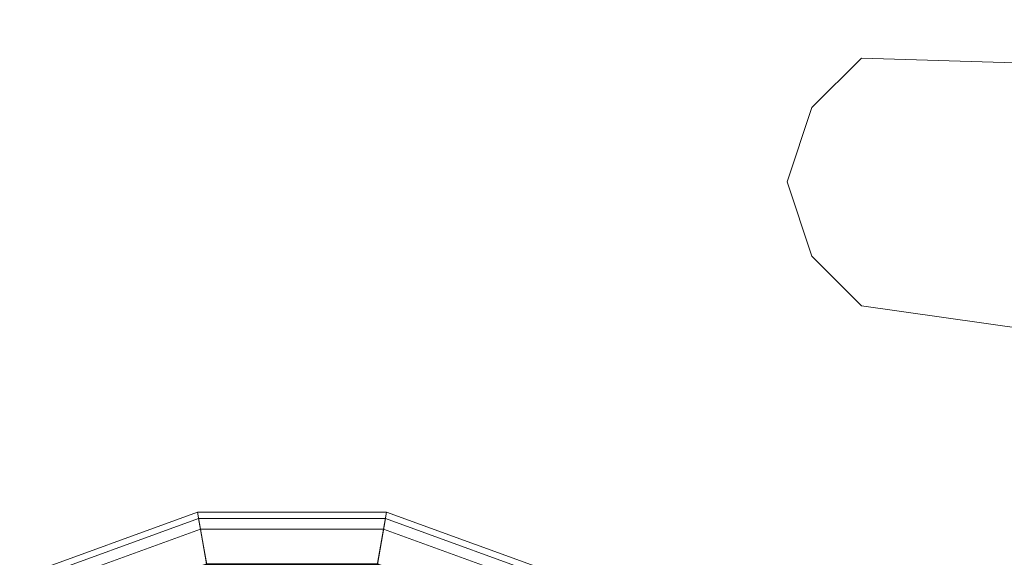
# Model space of a CAD drawing. Units: inches. Extents: x 375 to 1122, y 27 to 1069.
# Tile 34 of 155: x 732.385 to 734.833, y 282.464 to 283.8. Entities that reach past the tile are written whole.
import ezdxf

# ---------------------------------------------------------------- set-up
doc = ezdxf.new("R2010")
doc.units = ezdxf.units.IN
doc.layers.add('A-ANNO-DIMS', color=2, linetype='Continuous', lineweight=18)
doc.layers.add('Furniture', color=30, linetype='Continuous', lineweight=18)
doc.styles.get("Standard").update_dxf_attribs({"font": 'arial.ttf'})
doc.dimstyles.new('ISO-25', dxfattribs={"dimtxt": 12, "dimasz": 2.5, "dimexe": 1.5, "dimexo": 1.5, "dimtad": 1, "dimdec": 1, "dimlunit": 3, "dimtxsty": 'Standard', "dimblk": 'ARCHTICK', "dimcen": 2.5, "dimadec": 0, "dimazin": 0, "dimtfac": 1, "dimtdec": 1, "dimtmove": 0, "dimatfit": 3, "dimfxl": 1.5, "dimfxlon": 1, "dimarcsym": 0})

# ---------------------------------------------------------------- blocks, each defined once
blk = doc.blocks.new('A$C403C54AD')
for points, invisible_edges in [([(1.580288, 1.238319, -0.039653), (1.564897, 1.238319, -0.039653), (1.566436, 1.287573, -0.039653), (1.581828, 1.249093, -0.039653)], 5), ([(1.580288, 1.238319, -0.041193), (1.564897, 1.238319, -0.041193), (1.566436, 1.287573, -0.041193), (1.581828, 1.249093, -0.041193)], 5), ([(1.566436, 1.287573, -0.041193), (1.566436, 1.287573, -0.039653), (1.564897, 1.238319, -0.039653), (1.564897, 1.238319, -0.041193)], 5), ([(1.580288, 1.238319, -0.039653), (1.580288, 1.238319, -0.041193), (1.581828, 1.249093, -0.041193), (1.581828, 1.249093, -0.039653)], 5), ([(1.567975, 1.23524, -0.039653), (1.57721, 1.23524, -0.039653), (1.580288, 1.238319, -0.039653), (1.564897, 1.238319, -0.039653)], 5), ([(1.567975, 1.23524, -0.041193), (1.57721, 1.23524, -0.041193), (1.580288, 1.238319, -0.041193), (1.564897, 1.238319, -0.041193)], 5), ([(1.564897, 1.238319, -0.039653), (1.564897, 1.238319, -0.041193), (1.567975, 1.23524, -0.041193), (1.567975, 1.23524, -0.039653)], 5), ([(1.57721, 1.23524, -0.041193), (1.57721, 1.23524, -0.039653), (1.580288, 1.238319, -0.039653), (1.580288, 1.238319, -0.041193)], 5), ([(1.572592, 1.233701, -0.039653), (1.572592, 1.233701, -0.039653), (1.567975, 1.23524, -0.039653), (1.57721, 1.23524, -0.039653)], 4), ([(1.572592, 1.233701, -0.041193), (1.572592, 1.233701, -0.041193), (1.567975, 1.23524, -0.041193), (1.57721, 1.23524, -0.041193)], 4), ([(1.567975, 1.23524, -0.041193), (1.567975, 1.23524, -0.039653), (1.572592, 1.233701, -0.039653), (1.572592, 1.233701, -0.041193)], 1), ([(1.572592, 1.233701, -0.039653), (1.572592, 1.233701, -0.041193), (1.57721, 1.23524, -0.041193), (1.57721, 1.23524, -0.039653)], 4)]:
    blk.add_3dface(points, dxfattribs=dict(invisible_edges=invisible_edges))
for points in [[(1.597139, 1.219849, -0.04658), (1.626464, 1.202917, -0.043501), (1.626464, 1.202917, -0.043501), (1.593116, 1.208798, -0.04658)], [(1.599967, 1.218216, -0.043349), (1.597139, 1.219849, -0.04658), (1.593116, 1.208798, -0.04658), (1.596333, 1.20823, -0.043349)], [(1.600002, 1.218195, 0.116404), (1.597484, 1.219649, 0.10318), (1.593509, 1.208728, 0.10318), (1.596372, 1.208223, 0.116404)], [(1.597484, 1.219649, 0.10318), (1.598069, 1.219312, 0.074938), (1.594174, 1.208611, 0.074938), (1.593509, 1.208728, 0.10318)], [(1.598069, 1.219312, 0.074938), (1.602714, 1.216629, 0.056929), (1.599457, 1.20768, 0.056929), (1.594174, 1.208611, 0.074938)], [(1.593116, 1.208798, -0.04658), (1.626464, 1.202917, -0.043501), (1.626464, 1.202917, -0.043501), (1.593116, 1.197037, -0.04658)], [(1.596333, 1.20823, -0.043349), (1.593116, 1.208798, -0.04658), (1.593116, 1.197037, -0.04658), (1.596333, 1.197604, -0.043349)], [(1.596372, 1.208223, 0.116404), (1.593509, 1.208728, 0.10318), (1.593509, 1.197107, 0.10318), (1.596372, 1.197611, 0.116404)], [(1.593509, 1.208728, 0.10318), (1.594174, 1.208611, 0.074938), (1.594174, 1.197224, 0.074938), (1.593509, 1.197107, 0.10318)], [(1.594174, 1.208611, 0.074938), (1.599457, 1.20768, 0.056929), (1.599457, 1.198155, 0.056929), (1.594174, 1.197224, 0.074938)], [(1.593116, 1.197037, -0.04658), (1.626464, 1.202917, -0.043501), (1.626464, 1.202917, -0.043501), (1.597139, 1.185986, -0.04658)], [(1.594174, 1.197224, 0.074938), (1.599457, 1.198155, 0.056929), (1.602714, 1.189206, 0.056929), (1.598069, 1.186523, 0.074938)], [(1.596333, 1.197604, -0.043349), (1.593116, 1.197037, -0.04658), (1.597139, 1.185986, -0.04658), (1.599967, 1.187619, -0.043349)], [(1.596372, 1.197611, 0.116404), (1.593509, 1.197107, 0.10318), (1.597484, 1.186186, 0.10318), (1.600002, 1.187639, 0.116404)], [(1.593509, 1.197107, 0.10318), (1.594174, 1.197224, 0.074938), (1.598069, 1.186523, 0.074938), (1.597484, 1.186186, 0.10318)]]:
    blk.add_3dface(points)
blk = doc.blocks.new('_ArchTick')
at = {"color": 0, "linetype": 'ByBlock', "const_width": 0.15}
blk.add_lwpolyline([(-0.5, -0.5), (0.5, 0.5)], dxfattribs=at)
blk = doc.blocks.new('*D94')
at = {"layer": 'A-ANNO-DIMS', "color": 0, "lineweight": -2, "transparency": 16777216}
for p, q in [((734.0073, 117.5277), (734.0073, 114.5277)), ((773.0073, 117.5277), (773.0073, 114.5277)), ((734.0073, 116.0277), (773.0073, 116.0277))]:
    blk.add_line(p, q, dxfattribs=at)
at = {"layer": 'Defpoints', "color": 0, "transparency": 16777216}
for p in [(734.0073, 667.5277), (773.0073, 667.5277), (773.0073, 116.0277)]:
    blk.add_point(p, dxfattribs=at)
at = {"layer": 'A-ANNO-DIMS', "color": 0, "lineweight": -2, "transparency": 16777216, "xscale": 2.5, "yscale": 2.5, "zscale": 2.5, "rotation": 180}
blk.add_blockref('_ArchTick', (734.0073, 116.0277), dxfattribs=at)
at = {"layer": 'A-ANNO-DIMS', "color": 0, "lineweight": -2, "transparency": 16777216, "xscale": 2.5, "yscale": 2.5, "zscale": 2.5}
blk.add_blockref('_ArchTick', (773.0073, 116.0277), dxfattribs=at)
at = {"layer": 'A-ANNO-DIMS', "color": 0, "transparency": 16777216, "insert": (753.5073, 122.7837), "char_height": 12, "attachment_point": 5}
blk.add_mtext('3\'-3"', dxfattribs=at)

msp = doc.modelspace()

# ---------------------------------------------------------------- block references
at = {"layer": 'Furniture', "xscale": 39.9918517141215, "yscale": 39.9918517141215, "zscale": 39.9918517141215, "rotation": 270}
msp.add_blockref('A$C403C54AD', (684.9549, 346.2875, 0.024), dxfattribs=at)

# ---------------------------------------------------------------- dimensions: what is measured, and where the dimension line sits
at = {"layer": 'A-ANNO-DIMS'}
dim = msp.add_linear_dim(base=(773.0073, 116.0277), p1=(734.0073, 667.5277), p2=(773.0073, 667.5277), dimstyle='ISO-25', override={"dimdec": 1, "dimlfac": 1, "dimrnd": 0, "dimzin": 1, "dimdsep": 46, "dimlunit": 4, "dimfrac": 2}, dxfattribs=at)
dim.commit()
dim.dimension.update_dxf_attribs({"geometry": '*D94', "text_midpoint": (753.5073, 122.7837)})

doc.saveas('drawing.dxf')
